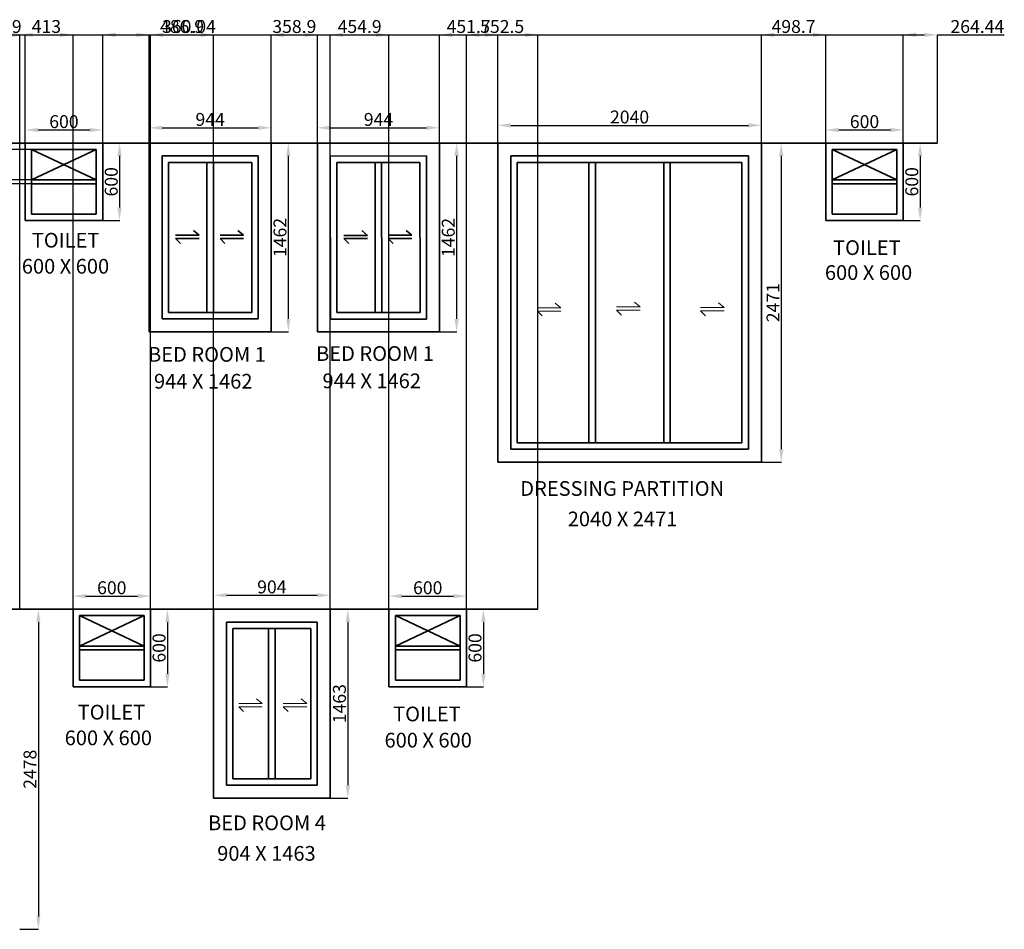
# Model space of a CAD drawing. Units: millimetres. Extents: x 5977 to 24120, y -1732 to 6209.
# Tile 3 of 3: x 16498 to 24120, y -1234 to 5807. Entities that reach past the tile are written whole.
import ezdxf

# ---------------------------------------------------------------- set-up
doc = ezdxf.new("R2010")
doc.units = ezdxf.units.MM
for name, color, linetype, lineweight in [('A-ANNO-DIMS', 2, 'Continuous', 18), ('A-ANNO-SYMB', 143, 'Continuous', 18), ('A-ANNO-TEXT', 7, 'Continuous', 25), ('A-GLAZ', 4, 'Continuous', 35)]:
    doc.layers.add(name, color=color, linetype=linetype, lineweight=lineweight)
doc.styles.get("Standard").update_dxf_attribs({"font": 'arial.ttf'})
doc.dimstyles.new('ISO-25', dxfattribs={"dimtxt": 100, "dimasz": 100, "dimexe": 1.25, "dimexo": 0.625, "dimtad": 1, "dimtxsty": 'Standard', "dimcen": 2.5, "dimadec": 0, "dimazin": 0, "dimtfac": 1, "dimtmove": 0, "dimatfit": 3, "dimfxl": 1, "dimarcsym": 0})

# ---------------------------------------------------------------- blocks, each defined once
blk = doc.blocks.new('*D11')
at = {"layer": 'A-ANNO-DIMS', "color": 0, "lineweight": -2, "transparency": 16777216}
for p, q in [((16540.9, 4852.8), (16540.9, 4954.6)), ((17140.9, 4852.8), (17140.9, 4954.6)), ((16640.9, 4953.4), (17040.9, 4953.4))]:
    blk.add_line(p, q, dxfattribs=at)
at = {"layer": 'A-ANNO-DIMS', "color": 0, "transparency": 16777216}
for points in [[(16640.9, 4970.1), (16640.9, 4936.7), (16540.9, 4953.4)], [(17040.9, 4970.1), (17040.9, 4936.7), (17140.9, 4953.4)]]:
    blk.add_solid(points, dxfattribs=at)
at = {"layer": 'Defpoints', "color": 0, "transparency": 16777216}
for p in [(17140.9, 4953.4), (16540.9, 4852.2), (17140.9, 4852.2)]:
    blk.add_point(p, dxfattribs=at)
at = {"layer": 'A-ANNO-DIMS', "color": 0, "transparency": 16777216, "insert": (16840.9, 5005.1), "char_height": 100, "attachment_point": 5}
blk.add_mtext('600', dxfattribs=at)
blk = doc.blocks.new('*D12')
at = {"layer": 'A-ANNO-DIMS', "color": 0, "lineweight": -2, "transparency": 16777216}
for p, q in [((17141.5, 4852.2), (17272.9, 4852.2)), ((17271.7, 4752.2), (17271.7, 4352.2)), ((17141.5, 4252.2), (17272.9, 4252.2))]:
    blk.add_line(p, q, dxfattribs=at)
at = {"layer": 'A-ANNO-DIMS', "color": 0, "transparency": 16777216}
for points in [[(17255, 4752.2), (17288.3, 4752.2), (17271.7, 4852.2)], [(17255, 4352.2), (17288.3, 4352.2), (17271.7, 4252.2)]]:
    blk.add_solid(points, dxfattribs=at)
at = {"layer": 'Defpoints', "color": 0, "transparency": 16777216}
for p in [(17140.9, 4852.2), (17140.9, 4252.2), (17271.7, 4252.2)]:
    blk.add_point(p, dxfattribs=at)
at = {"layer": 'A-ANNO-DIMS', "color": 0, "transparency": 16777216, "insert": (17220, 4552.2), "char_height": 100, "attachment_point": 5, "rotation": 90}
blk.add_mtext('600', dxfattribs=at)
blk = doc.blocks.new('*D13')
at = {"layer": 'A-ANNO-DIMS', "color": 0, "lineweight": -2, "transparency": 16777216}
for p, q in [((17500.9, 4852.8), (17500.9, 4971.3)), ((17600.9, 4970), (18344.9, 4970)), ((18444.9, 4852.8), (18444.9, 4971.3))]:
    blk.add_line(p, q, dxfattribs=at)
at = {"layer": 'A-ANNO-DIMS', "color": 0, "transparency": 16777216}
for points in [[(17600.9, 4986.7), (17600.9, 4953.4), (17500.9, 4970)], [(18344.9, 4986.7), (18344.9, 4953.4), (18444.9, 4970)]]:
    blk.add_solid(points, dxfattribs=at)
at = {"layer": 'Defpoints', "color": 0, "transparency": 16777216}
for p in [(18444.9, 4970), (17500.9, 4852.2), (18444.9, 4852.2)]:
    blk.add_point(p, dxfattribs=at)
at = {"layer": 'A-ANNO-DIMS', "color": 0, "transparency": 16777216, "insert": (17972.9, 5021.7), "char_height": 100, "attachment_point": 5}
blk.add_mtext('944', dxfattribs=at)
blk = doc.blocks.new('*D14')
at = {"layer": 'A-ANNO-DIMS', "color": 0, "lineweight": -2, "transparency": 16777216}
for p, q in [((18445.6, 4852.2), (18579.1, 4852.2)), ((18577.9, 4752.2), (18577.9, 3490.2)), ((18445.6, 3390.2), (18579.1, 3390.2))]:
    blk.add_line(p, q, dxfattribs=at)
at = {"layer": 'A-ANNO-DIMS', "color": 0, "transparency": 16777216}
for points in [[(18561.2, 4752.2), (18594.5, 4752.2), (18577.9, 4852.2)], [(18561.2, 3490.2), (18594.5, 3490.2), (18577.9, 3390.2)]]:
    blk.add_solid(points, dxfattribs=at)
at = {"layer": 'Defpoints', "color": 0, "transparency": 16777216}
for p in [(18444.9, 4852.2), (18444.9, 3390.2), (18577.9, 3390.2)]:
    blk.add_point(p, dxfattribs=at)
at = {"layer": 'A-ANNO-DIMS', "color": 0, "transparency": 16777216, "insert": (18526.2, 4121.2), "char_height": 100, "attachment_point": 5, "rotation": 90}
blk.add_mtext('1462', dxfattribs=at)
blk = doc.blocks.new('*D15')
at = {"layer": 'A-ANNO-DIMS', "color": 0, "lineweight": -2, "transparency": 16777216}
for p, q in [((18803.8, 4852.8), (18803.8, 4971.3)), ((18903.8, 4970), (19647.8, 4970)), ((19747.8, 4852.8), (19747.8, 4971.3))]:
    blk.add_line(p, q, dxfattribs=at)
at = {"layer": 'A-ANNO-DIMS', "color": 0, "transparency": 16777216}
for points in [[(18903.8, 4986.7), (18903.8, 4953.4), (18803.8, 4970)], [(19647.8, 4986.7), (19647.8, 4953.4), (19747.8, 4970)]]:
    blk.add_solid(points, dxfattribs=at)
at = {"layer": 'Defpoints', "color": 0, "transparency": 16777216}
for p in [(19747.8, 4970), (18803.8, 4852.2), (19747.8, 4852.2)]:
    blk.add_point(p, dxfattribs=at)
at = {"layer": 'A-ANNO-DIMS', "color": 0, "transparency": 16777216, "insert": (19275.8, 5021.7), "char_height": 100, "attachment_point": 5}
blk.add_mtext('944', dxfattribs=at)
blk = doc.blocks.new('*D16')
at = {"layer": 'A-ANNO-DIMS', "color": 0, "lineweight": -2, "transparency": 16777216}
for p, q in [((19748.5, 4852.2), (19882, 4852.2)), ((19880.8, 4752.2), (19880.8, 3490.2)), ((19748.5, 3390.2), (19882, 3390.2))]:
    blk.add_line(p, q, dxfattribs=at)
at = {"layer": 'A-ANNO-DIMS', "color": 0, "transparency": 16777216}
for points in [[(19864.1, 4752.2), (19897.4, 4752.2), (19880.8, 4852.2)], [(19864.1, 3490.2), (19897.4, 3490.2), (19880.8, 3390.2)]]:
    blk.add_solid(points, dxfattribs=at)
at = {"layer": 'Defpoints', "color": 0, "transparency": 16777216}
for p in [(19747.8, 4852.2), (19747.8, 3390.2), (19880.8, 3390.2)]:
    blk.add_point(p, dxfattribs=at)
at = {"layer": 'A-ANNO-DIMS', "color": 0, "transparency": 16777216, "insert": (19829.1, 4121.2), "char_height": 100, "attachment_point": 5, "rotation": 90}
blk.add_mtext('1462', dxfattribs=at)
blk = doc.blocks.new('*D17')
at = {"layer": 'A-ANNO-DIMS', "color": 0, "lineweight": -2, "transparency": 16777216}
for p, q in [((20199.5, 4852.8), (20199.5, 4990.3)), ((20299.5, 4989), (22139.5, 4989)), ((22239.5, 4852.8), (22239.5, 4990.3))]:
    blk.add_line(p, q, dxfattribs=at)
at = {"layer": 'A-ANNO-DIMS', "color": 0, "transparency": 16777216}
for points in [[(20299.5, 5005.7), (20299.5, 4972.4), (20199.5, 4989)], [(22139.5, 5005.7), (22139.5, 4972.4), (22239.5, 4989)]]:
    blk.add_solid(points, dxfattribs=at)
at = {"layer": 'Defpoints', "color": 0, "transparency": 16777216}
for p in [(22239.5, 4989), (20199.5, 4852.2), (22239.5, 4852.2)]:
    blk.add_point(p, dxfattribs=at)
at = {"layer": 'A-ANNO-DIMS', "color": 0, "transparency": 16777216, "insert": (21219.5, 5040.7), "char_height": 100, "attachment_point": 5}
blk.add_mtext('2040', dxfattribs=at)
blk = doc.blocks.new('*D18')
at = {"layer": 'A-ANNO-DIMS', "color": 0, "lineweight": -2, "transparency": 16777216}
for p, q in [((22240.1, 4852.2), (22394.9, 4852.2)), ((22393.6, 4752.2), (22393.6, 2481.2)), ((22240.1, 2381.2), (22394.9, 2381.2))]:
    blk.add_line(p, q, dxfattribs=at)
at = {"layer": 'A-ANNO-DIMS', "color": 0, "transparency": 16777216}
for points in [[(22377, 4752.2), (22410.3, 4752.2), (22393.6, 4852.2)], [(22377, 2481.2), (22410.3, 2481.2), (22393.6, 2381.2)]]:
    blk.add_solid(points, dxfattribs=at)
at = {"layer": 'Defpoints', "color": 0, "transparency": 16777216}
for p in [(22239.5, 4852.2), (22239.5, 2381.2), (22393.6, 2381.2)]:
    blk.add_point(p, dxfattribs=at)
at = {"layer": 'A-ANNO-DIMS', "color": 0, "transparency": 16777216, "insert": (22342.8, 3616.7), "char_height": 100, "attachment_point": 5, "rotation": 90}
blk.add_mtext('2471', dxfattribs=at)
blk = doc.blocks.new('*D19')
at = {"layer": 'A-ANNO-DIMS', "color": 0, "lineweight": -2, "transparency": 16777216}
for p, q in [((22738.2, 4852.8), (22738.2, 4954.6)), ((23338.2, 4852.8), (23338.2, 4954.6)), ((22838.2, 4953.4), (23238.2, 4953.4))]:
    blk.add_line(p, q, dxfattribs=at)
at = {"layer": 'A-ANNO-DIMS', "color": 0, "transparency": 16777216}
for points in [[(22838.2, 4970.1), (22838.2, 4936.7), (22738.2, 4953.4)], [(23238.2, 4970.1), (23238.2, 4936.7), (23338.2, 4953.4)]]:
    blk.add_solid(points, dxfattribs=at)
at = {"layer": 'Defpoints', "color": 0, "transparency": 16777216}
for p in [(23338.2, 4953.4), (22738.2, 4852.2), (23338.2, 4852.2)]:
    blk.add_point(p, dxfattribs=at)
at = {"layer": 'A-ANNO-DIMS', "color": 0, "transparency": 16777216, "insert": (23038.2, 5005.1), "char_height": 100, "attachment_point": 5}
blk.add_mtext('600', dxfattribs=at)
blk = doc.blocks.new('*D20')
at = {"layer": 'A-ANNO-DIMS', "color": 0, "lineweight": -2, "transparency": 16777216}
for p, q in [((23338.8, 4852.2), (23470.2, 4852.2)), ((23468.9, 4752.2), (23468.9, 4352.2)), ((23338.8, 4252.2), (23470.2, 4252.2))]:
    blk.add_line(p, q, dxfattribs=at)
at = {"layer": 'A-ANNO-DIMS', "color": 0, "transparency": 16777216}
for points in [[(23452.3, 4752.2), (23485.6, 4752.2), (23468.9, 4852.2)], [(23452.3, 4352.2), (23485.6, 4352.2), (23468.9, 4252.2)]]:
    blk.add_solid(points, dxfattribs=at)
at = {"layer": 'Defpoints', "color": 0, "transparency": 16777216}
for p in [(23338.2, 4852.2), (23338.2, 4252.2), (23468.9, 4252.2)]:
    blk.add_point(p, dxfattribs=at)
at = {"layer": 'A-ANNO-DIMS', "color": 0, "transparency": 16777216, "insert": (23417.2, 4552.2), "char_height": 100, "attachment_point": 5, "rotation": 90}
blk.add_mtext('600', dxfattribs=at)
blk = doc.blocks.new('*D25')
at = {"layer": 'A-ANNO-DIMS', "color": 0, "lineweight": -2, "transparency": 16777216}
for p, q in [((16911.4, 1244.3), (16911.4, 1346.1)), ((17011.4, 1344.9), (17411.4, 1344.9)), ((17511.4, 1244.3), (17511.4, 1346.1))]:
    blk.add_line(p, q, dxfattribs=at)
at = {"layer": 'A-ANNO-DIMS', "color": 0, "transparency": 16777216}
for points in [[(17011.4, 1361.5), (17011.4, 1328.2), (16911.4, 1344.9)], [(17411.4, 1361.5), (17411.4, 1328.2), (17511.4, 1344.9)]]:
    blk.add_solid(points, dxfattribs=at)
at = {"layer": 'Defpoints', "color": 0, "transparency": 16777216}
for p in [(17511.4, 1344.9), (16911.4, 1243.7), (17511.4, 1243.7)]:
    blk.add_point(p, dxfattribs=at)
at = {"layer": 'A-ANNO-DIMS', "color": 0, "transparency": 16777216, "insert": (17211.4, 1396.6), "char_height": 100, "attachment_point": 5}
blk.add_mtext('600', dxfattribs=at)
blk = doc.blocks.new('*D26')
at = {"layer": 'A-ANNO-DIMS', "color": 0, "lineweight": -2, "transparency": 16777216}
for p, q in [((17512.1, 1243.7), (17643.4, 1243.7)), ((17642.2, 1143.7), (17642.2, 743.7)), ((17512.1, 643.7), (17643.4, 643.7))]:
    blk.add_line(p, q, dxfattribs=at)
at = {"layer": 'A-ANNO-DIMS', "color": 0, "transparency": 16777216}
for points in [[(17625.5, 1143.7), (17658.9, 1143.7), (17642.2, 1243.7)], [(17625.5, 743.7), (17658.9, 743.7), (17642.2, 643.7)]]:
    blk.add_solid(points, dxfattribs=at)
at = {"layer": 'Defpoints', "color": 0, "transparency": 16777216}
for p in [(17511.4, 1243.7), (17511.4, 643.7), (17642.2, 643.7)]:
    blk.add_point(p, dxfattribs=at)
at = {"layer": 'A-ANNO-DIMS', "color": 0, "transparency": 16777216, "insert": (17590.5, 943.7), "char_height": 100, "attachment_point": 5, "rotation": 90}
blk.add_mtext('600', dxfattribs=at)
blk = doc.blocks.new('*D32')
at = {"layer": 'A-ANNO-DIMS', "color": 0, "lineweight": -2, "transparency": 16777216}
for p, q in [((16499.1, 1243.7), (16644.2, 1243.7)), ((16643, 1143.7), (16643, -1134.3)), ((16499.1, -1234.3), (16644.2, -1234.3))]:
    blk.add_line(p, q, dxfattribs=at)
at = {"layer": 'A-ANNO-DIMS', "color": 0, "transparency": 16777216}
for points in [[(16626.3, 1143.7), (16659.6, 1143.7), (16643, 1243.7)], [(16626.3, -1134.3), (16659.6, -1134.3), (16643, -1234.3)]]:
    blk.add_solid(points, dxfattribs=at)
at = {"layer": 'Defpoints', "color": 0, "transparency": 16777216}
for p in [(16498.5, 1243.7), (16498.5, -1234.3), (16643, -1234.3)]:
    blk.add_point(p, dxfattribs=at)
at = {"layer": 'A-ANNO-DIMS', "color": 0, "transparency": 16777216, "insert": (16591.3, 4.7), "char_height": 100, "attachment_point": 5, "rotation": 90}
blk.add_mtext('2478', dxfattribs=at)
blk = doc.blocks.new('*D33')
at = {"layer": 'A-ANNO-DIMS', "color": 0, "lineweight": -2, "transparency": 16777216}
for p, q in [((17998.3, 1244.3), (17998.3, 1352.8)), ((18098.3, 1351.6), (18802.3, 1351.6)), ((18902.3, 1244.3), (18902.3, 1352.8))]:
    blk.add_line(p, q, dxfattribs=at)
at = {"layer": 'A-ANNO-DIMS', "color": 0, "transparency": 16777216}
for points in [[(18098.3, 1368.3), (18098.3, 1334.9), (17998.3, 1351.6)], [(18802.3, 1368.3), (18802.3, 1334.9), (18902.3, 1351.6)]]:
    blk.add_solid(points, dxfattribs=at)
at = {"layer": 'Defpoints', "color": 0, "transparency": 16777216}
for p in [(18902.3, 1351.6), (17998.3, 1243.7), (18902.3, 1243.7)]:
    blk.add_point(p, dxfattribs=at)
at = {"layer": 'A-ANNO-DIMS', "color": 0, "transparency": 16777216, "insert": (18450.3, 1403.3), "char_height": 100, "attachment_point": 5}
blk.add_mtext('904', dxfattribs=at)
blk = doc.blocks.new('*D34')
at = {"layer": 'A-ANNO-DIMS', "color": 0, "lineweight": -2, "transparency": 16777216}
for p, q in [((18902.9, 1243.7), (19039.7, 1243.7)), ((19038.4, 1143.7), (19038.4, -119.3)), ((18902.9, -219.3), (19039.7, -219.3))]:
    blk.add_line(p, q, dxfattribs=at)
at = {"layer": 'A-ANNO-DIMS', "color": 0, "transparency": 16777216}
for points in [[(19021.7, 1143.7), (19055.1, 1143.7), (19038.4, 1243.7)], [(19021.7, -119.3), (19055.1, -119.3), (19038.4, -219.3)]]:
    blk.add_solid(points, dxfattribs=at)
at = {"layer": 'Defpoints', "color": 0, "transparency": 16777216}
for p in [(18902.3, 1243.7), (18902.3, -219.3), (19038.4, -219.3)]:
    blk.add_point(p, dxfattribs=at)
at = {"layer": 'A-ANNO-DIMS', "color": 0, "transparency": 16777216, "insert": (18986.7, 512.2), "char_height": 100, "attachment_point": 5, "rotation": 90}
blk.add_mtext('1463', dxfattribs=at)
blk = doc.blocks.new('*D35')
at = {"layer": 'A-ANNO-DIMS', "color": 0, "lineweight": -2, "transparency": 16777216}
for p, q in [((19357.2, 1244.3), (19357.2, 1346.1)), ((19457.2, 1344.9), (19857.2, 1344.9)), ((19957.2, 1244.3), (19957.2, 1346.1))]:
    blk.add_line(p, q, dxfattribs=at)
at = {"layer": 'A-ANNO-DIMS', "color": 0, "transparency": 16777216}
for points in [[(19457.2, 1361.5), (19457.2, 1328.2), (19357.2, 1344.9)], [(19857.2, 1361.5), (19857.2, 1328.2), (19957.2, 1344.9)]]:
    blk.add_solid(points, dxfattribs=at)
at = {"layer": 'Defpoints', "color": 0, "transparency": 16777216}
for p in [(19957.2, 1344.9), (19357.2, 1243.7), (19957.2, 1243.7)]:
    blk.add_point(p, dxfattribs=at)
at = {"layer": 'A-ANNO-DIMS', "color": 0, "transparency": 16777216, "insert": (19657.2, 1396.6), "char_height": 100, "attachment_point": 5}
blk.add_mtext('600', dxfattribs=at)
blk = doc.blocks.new('*D36')
at = {"layer": 'A-ANNO-DIMS', "color": 0, "lineweight": -2, "transparency": 16777216}
for p, q in [((19957.9, 1243.7), (20089.2, 1243.7)), ((20088, 1143.7), (20088, 743.7)), ((19957.9, 643.7), (20089.2, 643.7))]:
    blk.add_line(p, q, dxfattribs=at)
at = {"layer": 'A-ANNO-DIMS', "color": 0, "transparency": 16777216}
for points in [[(20071.3, 1143.7), (20104.7, 1143.7), (20088, 1243.7)], [(20071.3, 743.7), (20104.7, 743.7), (20088, 643.7)]]:
    blk.add_solid(points, dxfattribs=at)
at = {"layer": 'Defpoints', "color": 0, "transparency": 16777216}
for p in [(19957.2, 1243.7), (19957.2, 643.7), (20088, 643.7)]:
    blk.add_point(p, dxfattribs=at)
at = {"layer": 'A-ANNO-DIMS', "color": 0, "transparency": 16777216, "insert": (20036.3, 943.7), "char_height": 100, "attachment_point": 5, "rotation": 90}
blk.add_mtext('600', dxfattribs=at)
blk = doc.blocks.new('WIN-600x600-TOILET')
for p, q in [((16540.9, 4852.2), (16540.9, 4252.2)), ((16590.9, 4802.2), (16590.9, 4302.2)), ((16590.9, 4802.2), (17090.9, 4802.2)), ((16590.9, 4567.2), (17090.9, 4802.2)), ((17090.9, 4567.2), (16590.9, 4802.2)), ((17090.9, 4302.2), (17090.9, 4802.2)), ((17140.9, 4252.2), (17140.9, 4852.2)), ((16590.9, 4567.2), (17090.9, 4567.2)), ((16590.9, 4302.2), (17090.9, 4302.2)), ((16540.9, 4252.2), (17140.9, 4252.2))]:
    blk.add_line(p, q)
blk = doc.blocks.new('WIN-944x1462-BED')
for p, q in [((17600.9, 4752.2), (18344.9, 4752.2)), ((17600.9, 4752.2), (17600.9, 3490.2)), ((18344.9, 3490.2), (18344.9, 4752.2)), ((17650.9, 4702.2), (18294.9, 4702.2)), ((17650.9, 4702.2), (17650.9, 3540.2)), ((17947.9, 4702.2), (17947.9, 3540.2)), ((17997.9, 4702.2), (17997.9, 3540.2)), ((18294.9, 3540.2), (18294.9, 4702.2)), ((17705.1, 4138.2), (17887.8, 4138.2)), ((17887.8, 4138.2), (17843.7, 4175.4)), ((18049.1, 4138.2), (18231.8, 4138.2)), ((18231.8, 4138.2), (18187.7, 4175.4)), ((17705, 4113), (17887.4, 4113)), ((17705, 4113), (17742.7, 4075.4)), ((18049.1, 4113), (18231.4, 4113)), ((18049.1, 4113), (18086.7, 4075.4)), ((17650.9, 3540.2), (18294.9, 3540.2)), ((17600.9, 3490.2), (18344.9, 3490.2))]:
    blk.add_line(p, q)
blk = doc.blocks.new('ARROW-SLIDE')
for p, q in [((14721.8, 21.3), (14904.6, 21.3)), ((14904.6, 21.3), (14860.5, 58.6)), ((14721.8, -3.8), (14904.1, -3.8)), ((14721.8, -3.8), (14759.4, -41.4))]:
    blk.add_line(p, q)
blk = doc.blocks.new('*D41')
at = {"layer": 'A-ANNO-DIMS', "color": 0, "lineweight": -2, "transparency": 16777216}
for p, q in [((6975.8, 4852.8), (6975.8, 5690.9)), ((7075.8, 5689.7), (23502.6, 5689.7)), ((23602.6, 4852.8), (23602.6, 5690.9))]:
    blk.add_line(p, q, dxfattribs=at)
at = {"layer": 'A-ANNO-DIMS', "color": 0, "transparency": 16777216}
for points in [[(7075.8, 5706.3), (7075.8, 5673), (6975.8, 5689.7)], [(23502.6, 5706.3), (23502.6, 5673), (23602.6, 5689.7)]]:
    blk.add_solid(points, dxfattribs=at)
at = {"layer": 'Defpoints', "color": 0, "transparency": 16777216}
for p in [(23602.6, 5689.7), (6975.8, 4852.2), (23602.6, 4852.2)]:
    blk.add_point(p, dxfattribs=at)
at = {"layer": 'A-ANNO-DIMS', "color": 0, "transparency": 16777216, "insert": (15289.2, 5741.3), "char_height": 100, "attachment_point": 5}
blk.add_mtext('16627', dxfattribs=at)
blk = doc.blocks.new('*D42')
at = {"layer": 'A-ANNO-DIMS', "color": 0, "lineweight": -2, "transparency": 16777216}
for p, q in [((6931.9, 1244.3), (6931.9, 5690.9)), ((7031.9, 5689.7), (20409.7, 5689.7)), ((20509.7, 1244.3), (20509.7, 5690.9))]:
    blk.add_line(p, q, dxfattribs=at)
at = {"layer": 'A-ANNO-DIMS', "color": 0, "transparency": 16777216}
for points in [[(7031.9, 5706.3), (7031.9, 5673), (6931.9, 5689.7)], [(20409.7, 5706.3), (20409.7, 5673), (20509.7, 5689.7)]]:
    blk.add_solid(points, dxfattribs=at)
at = {"layer": 'Defpoints', "color": 0, "transparency": 16777216}
for p in [(20509.7, 5689.7), (6931.9, 1243.7), (20509.7, 1243.7)]:
    blk.add_point(p, dxfattribs=at)
at = {"layer": 'A-ANNO-DIMS', "color": 0, "transparency": 16777216, "insert": (13720.8, 5741.4), "char_height": 100, "attachment_point": 5}
blk.add_mtext('13578', dxfattribs=at)
blk = doc.blocks.new('*D48')
at = {"layer": 'A-ANNO-DIMS', "color": 0, "lineweight": -2, "transparency": 16777216}
for p, q in [((16145, 4852.8), (16145, 5690.9)), ((16245, 5689.7), (16440.9, 5689.7)), ((16540.9, 4852.8), (16540.9, 5690.9))]:
    blk.add_line(p, q, dxfattribs=at)
at = {"layer": 'A-ANNO-DIMS', "color": 0, "transparency": 16777216}
for points in [[(16245, 5706.3), (16245, 5673), (16145, 5689.7)], [(16440.9, 5706.3), (16440.9, 5673), (16540.9, 5689.7)]]:
    blk.add_solid(points, dxfattribs=at)
at = {"layer": 'Defpoints', "color": 0, "transparency": 16777216}
for p in [(16540.9, 5689.7), (16145, 4852.2), (16540.9, 4852.2)]:
    blk.add_point(p, dxfattribs=at)
at = {"layer": 'A-ANNO-DIMS', "color": 0, "transparency": 16777216, "insert": (16343, 5741.4), "char_height": 100, "attachment_point": 5}
blk.add_mtext('395.9', dxfattribs=at)
blk = doc.blocks.new('*D49')
at = {"layer": 'A-ANNO-DIMS', "color": 0, "lineweight": -2, "transparency": 16777216}
for p, q in [((17140.9, 4852.8), (17140.9, 5690.9)), ((17240.9, 5689.7), (17400.9, 5689.7)), ((17500.9, 4852.8), (17500.9, 5690.9)), ((17500.9, 5689.7), (18016.9, 5689.7))]:
    blk.add_line(p, q, dxfattribs=at)
at = {"layer": 'A-ANNO-DIMS', "color": 0, "transparency": 16777216}
for points in [[(17240.9, 5706.3), (17240.9, 5673), (17140.9, 5689.7)], [(17400.9, 5706.3), (17400.9, 5673), (17500.9, 5689.7)]]:
    blk.add_solid(points, dxfattribs=at)
at = {"layer": 'Defpoints', "color": 0, "transparency": 16777216}
for p in [(17500.9, 5689.7), (17140.9, 4852.2), (17500.9, 4852.2)]:
    blk.add_point(p, dxfattribs=at)
at = {"layer": 'A-ANNO-DIMS', "color": 0, "transparency": 16777216, "insert": (17808.9, 5741.4), "char_height": 100, "attachment_point": 5}
blk.add_mtext('360.04', dxfattribs=at)
blk = doc.blocks.new('*D50')
at = {"layer": 'A-ANNO-DIMS', "color": 0, "lineweight": -2, "transparency": 16777216}
for p, q in [((18444.9, 4852.8), (18444.9, 5690.9)), ((18544.9, 5689.7), (18703.8, 5689.7)), ((18803.8, 4852.8), (18803.8, 5690.9))]:
    blk.add_line(p, q, dxfattribs=at)
at = {"layer": 'A-ANNO-DIMS', "color": 0, "transparency": 16777216}
for points in [[(18544.9, 5706.3), (18544.9, 5673), (18444.9, 5689.7)], [(18703.8, 5706.3), (18703.8, 5673), (18803.8, 5689.7)]]:
    blk.add_solid(points, dxfattribs=at)
at = {"layer": 'Defpoints', "color": 0, "transparency": 16777216}
for p in [(18803.8, 5689.7), (18444.9, 4852.2), (18803.8, 4852.2)]:
    blk.add_point(p, dxfattribs=at)
at = {"layer": 'A-ANNO-DIMS', "color": 0, "transparency": 16777216, "insert": (18624.4, 5741.4), "char_height": 100, "attachment_point": 5}
blk.add_mtext('358.9', dxfattribs=at)
blk = doc.blocks.new('*D51')
at = {"layer": 'A-ANNO-DIMS', "color": 0, "lineweight": -2, "transparency": 16777216}
for p, q in [((19747.8, 4852.8), (19747.8, 5690.9)), ((19847.8, 5689.7), (20099.5, 5689.7)), ((20199.5, 4852.8), (20199.5, 5690.9))]:
    blk.add_line(p, q, dxfattribs=at)
at = {"layer": 'A-ANNO-DIMS', "color": 0, "transparency": 16777216}
for points in [[(19847.8, 5706.3), (19847.8, 5673), (19747.8, 5689.7)], [(20099.5, 5706.3), (20099.5, 5673), (20199.5, 5689.7)]]:
    blk.add_solid(points, dxfattribs=at)
at = {"layer": 'Defpoints', "color": 0, "transparency": 16777216}
for p in [(20199.5, 5689.7), (19747.8, 4852.2), (20199.5, 4852.2)]:
    blk.add_point(p, dxfattribs=at)
at = {"layer": 'A-ANNO-DIMS', "color": 0, "transparency": 16777216, "insert": (19973.7, 5741.3), "char_height": 100, "attachment_point": 5}
blk.add_mtext('451.7', dxfattribs=at)
blk = doc.blocks.new('*D52')
at = {"layer": 'A-ANNO-DIMS', "color": 0, "lineweight": -2, "transparency": 16777216}
for p, q in [((22239.5, 4852.8), (22239.5, 5690.9)), ((22339.5, 5689.7), (22638.2, 5689.7)), ((22738.2, 4852.8), (22738.2, 5690.9))]:
    blk.add_line(p, q, dxfattribs=at)
at = {"layer": 'A-ANNO-DIMS', "color": 0, "transparency": 16777216}
for points in [[(22339.5, 5706.3), (22339.5, 5673), (22239.5, 5689.7)], [(22638.2, 5706.3), (22638.2, 5673), (22738.2, 5689.7)]]:
    blk.add_solid(points, dxfattribs=at)
at = {"layer": 'Defpoints', "color": 0, "transparency": 16777216}
for p in [(22738.2, 5689.7), (22239.5, 4852.2), (22738.2, 4852.2)]:
    blk.add_point(p, dxfattribs=at)
at = {"layer": 'A-ANNO-DIMS', "color": 0, "transparency": 16777216, "insert": (22488.8, 5741.3), "char_height": 100, "attachment_point": 5}
blk.add_mtext('498.7', dxfattribs=at)
blk = doc.blocks.new('*D53')
at = {"layer": 'A-ANNO-DIMS', "color": 0, "lineweight": -2, "transparency": 16777216}
for p, q in [((23338.2, 4852.8), (23338.2, 5690.9)), ((23438.2, 5689.7), (23502.6, 5689.7)), ((23602.6, 4852.8), (23602.6, 5690.9)), ((23602.6, 5689.7), (24120.3, 5689.7))]:
    blk.add_line(p, q, dxfattribs=at)
at = {"layer": 'A-ANNO-DIMS', "color": 0, "transparency": 16777216}
for points in [[(23438.2, 5706.3), (23438.2, 5673), (23338.2, 5689.7)], [(23502.6, 5706.3), (23502.6, 5673), (23602.6, 5689.7)]]:
    blk.add_solid(points, dxfattribs=at)
at = {"layer": 'Defpoints', "color": 0, "transparency": 16777216}
for p in [(23602.6, 5689.7), (23338.2, 4852.2), (23602.6, 4852.2)]:
    blk.add_point(p, dxfattribs=at)
at = {"layer": 'A-ANNO-DIMS', "color": 0, "transparency": 16777216, "insert": (23911.5, 5741.3), "char_height": 100, "attachment_point": 5}
blk.add_mtext('264.44', dxfattribs=at)
blk = doc.blocks.new('*D57')
at = {"layer": 'A-ANNO-DIMS', "color": 0, "lineweight": -2, "transparency": 16777216}
for p, q in [((16498.5, 1244.3), (16498.5, 5690.9)), ((16598.5, 5689.7), (16811.4, 5689.7)), ((16911.4, 1244.3), (16911.4, 5690.9))]:
    blk.add_line(p, q, dxfattribs=at)
at = {"layer": 'A-ANNO-DIMS', "color": 0, "transparency": 16777216}
for points in [[(16598.5, 5706.3), (16598.5, 5673), (16498.5, 5689.7)], [(16811.4, 5706.3), (16811.4, 5673), (16911.4, 5689.7)]]:
    blk.add_solid(points, dxfattribs=at)
at = {"layer": 'Defpoints', "color": 0, "transparency": 16777216}
for p in [(16911.4, 5689.7), (16498.5, 1243.7), (16911.4, 1243.7)]:
    blk.add_point(p, dxfattribs=at)
at = {"layer": 'A-ANNO-DIMS', "color": 0, "transparency": 16777216, "insert": (16705, 5741.4), "char_height": 100, "attachment_point": 5}
blk.add_mtext('413', dxfattribs=at)
blk = doc.blocks.new('*D58')
at = {"layer": 'A-ANNO-DIMS', "color": 0, "lineweight": -2, "transparency": 16777216}
for p, q in [((17511.4, 1244.3), (17511.4, 5690.9)), ((17611.4, 5689.7), (17898.3, 5689.7)), ((17998.3, 1244.3), (17998.3, 5690.9))]:
    blk.add_line(p, q, dxfattribs=at)
at = {"layer": 'A-ANNO-DIMS', "color": 0, "transparency": 16777216}
for points in [[(17611.4, 5706.3), (17611.4, 5673), (17511.4, 5689.7)], [(17898.3, 5706.3), (17898.3, 5673), (17998.3, 5689.7)]]:
    blk.add_solid(points, dxfattribs=at)
at = {"layer": 'Defpoints', "color": 0, "transparency": 16777216}
for p in [(17998.3, 5689.7), (17511.4, 1243.7), (17998.3, 1243.7)]:
    blk.add_point(p, dxfattribs=at)
at = {"layer": 'A-ANNO-DIMS', "color": 0, "transparency": 16777216, "insert": (17754.9, 5741.3), "char_height": 100, "attachment_point": 5}
blk.add_mtext('486.9', dxfattribs=at)
blk = doc.blocks.new('*D59')
at = {"layer": 'A-ANNO-DIMS', "color": 0, "lineweight": -2, "transparency": 16777216}
for p, q in [((18902.3, 1244.3), (18902.3, 5690.9)), ((19002.3, 5689.7), (19257.2, 5689.7)), ((19357.2, 1244.3), (19357.2, 5690.9))]:
    blk.add_line(p, q, dxfattribs=at)
at = {"layer": 'A-ANNO-DIMS', "color": 0, "transparency": 16777216}
for points in [[(19002.3, 5706.3), (19002.3, 5673), (18902.3, 5689.7)], [(19257.2, 5706.3), (19257.2, 5673), (19357.2, 5689.7)]]:
    blk.add_solid(points, dxfattribs=at)
at = {"layer": 'Defpoints', "color": 0, "transparency": 16777216}
for p in [(19357.2, 5689.7), (18902.3, 1243.7), (19357.2, 1243.7)]:
    blk.add_point(p, dxfattribs=at)
at = {"layer": 'A-ANNO-DIMS', "color": 0, "transparency": 16777216, "insert": (19129.8, 5741.3), "char_height": 100, "attachment_point": 5}
blk.add_mtext('454.9', dxfattribs=at)
blk = doc.blocks.new('*D60')
at = {"layer": 'A-ANNO-DIMS', "color": 0, "lineweight": -2, "transparency": 16777216}
for p, q in [((19957.2, 1244.3), (19957.2, 5690.9)), ((20057.2, 5689.7), (20409.7, 5689.7)), ((20509.7, 1244.3), (20509.7, 5690.9))]:
    blk.add_line(p, q, dxfattribs=at)
at = {"layer": 'A-ANNO-DIMS', "color": 0, "transparency": 16777216}
for points in [[(20057.2, 5706.3), (20057.2, 5673), (19957.2, 5689.7)], [(20409.7, 5706.3), (20409.7, 5673), (20509.7, 5689.7)]]:
    blk.add_solid(points, dxfattribs=at)
at = {"layer": 'Defpoints', "color": 0, "transparency": 16777216}
for p in [(20509.7, 5689.7), (19957.2, 1243.7), (20509.7, 1243.7)]:
    blk.add_point(p, dxfattribs=at)
at = {"layer": 'A-ANNO-DIMS', "color": 0, "transparency": 16777216, "insert": (20233.5, 5741.3), "char_height": 100, "attachment_point": 5}
blk.add_mtext('552.5', dxfattribs=at)
blk = doc.blocks.new('*D67')
at = {"layer": 'A-ANNO-DIMS', "color": 0, "lineweight": -2, "transparency": 16777216}
for p, q in [((16590.3, 4802.2), (6093.2, 4802.2)), ((6094.4, 4702.2), (6094.4, 4667.2)), ((16590.3, 4567.2), (6093.2, 4567.2))]:
    blk.add_line(p, q, dxfattribs=at)
at = {"layer": 'A-ANNO-DIMS', "color": 0, "transparency": 16777216}
for points in [[(6077.8, 4702.2), (6111.1, 4702.2), (6094.4, 4802.2)], [(6077.8, 4667.2), (6111.1, 4667.2), (6094.4, 4567.2)]]:
    blk.add_solid(points, dxfattribs=at)
at = {"layer": 'Defpoints', "color": 0, "transparency": 16777216}
for p in [(16590.9, 4802.2), (6094.4, 4567.2), (16590.9, 4567.2)]:
    blk.add_point(p, dxfattribs=at)
at = {"layer": 'A-ANNO-DIMS', "color": 0, "transparency": 16777216, "insert": (6042.7, 4684.7), "char_height": 100, "attachment_point": 5, "rotation": 90}
blk.add_mtext('235', dxfattribs=at)
blk = doc.blocks.new('*D68')
at = {"layer": 'A-ANNO-DIMS', "color": 0, "lineweight": -2, "transparency": 16777216}
for p, q in [((6094.4, 4667.2), (6094.4, 4767.2)), ((16590.3, 4567.2), (6093.2, 4567.2)), ((16590.3, 4537.2), (6093.2, 4537.2)), ((6094.4, 4567.2), (6094.4, 4537.2)), ((6094.4, 4437.2), (6094.4, 4193.1))]:
    blk.add_line(p, q, dxfattribs=at)
at = {"layer": 'A-ANNO-DIMS', "color": 0, "transparency": 16777216}
for points in [[(6077.8, 4667.2), (6111.1, 4667.2), (6094.4, 4567.2)], [(6077.8, 4437.2), (6111.1, 4437.2), (6094.4, 4537.2)]]:
    blk.add_solid(points, dxfattribs=at)
at = {"layer": 'Defpoints', "color": 0, "transparency": 16777216}
for p in [(6094.4, 4537.2), (16590.9, 4567.2), (16590.9, 4537.2)]:
    blk.add_point(p, dxfattribs=at)
at = {"layer": 'A-ANNO-DIMS', "color": 0, "transparency": 16777216, "insert": (6042.7, 4265.1), "char_height": 100, "attachment_point": 5, "rotation": 90}
blk.add_mtext('30', dxfattribs=at)

msp = doc.modelspace()

# ---------------------------------------------------------------- linework, layer by layer
at = {"layer": 'A-GLAZ'}
for p, q in [((6975.757, 4852.16), (19747.827, 4852.16)), ((17500.947, 4852.16), (17500.947, 3390.16)), ((18444.947, 3390.16), (18444.947, 4852.16)), ((18803.827, 4852.16), (18803.827, 3390.16)), ((19747.827, 3390.16), (19747.827, 4852.16)), ((19747.827, 4852.16), (23602.612, 4852.16)), ((20199.487, 4852.16), (20199.487, 2381.16)), ((22239.487, 2381.16), (22239.487, 4852.16)), ((20299.487, 4752.16), (20299.487, 2481.16)), ((20299.487, 4752.16), (22139.487, 4752.16)), ((22139.487, 2481.16), (22139.487, 4752.16)), ((20349.487, 4702.16), (20349.487, 2531.16)), ((20349.487, 4702.16), (22089.487, 4702.16)), ((20904.487, 4702.16), (20904.487, 2531.16)), ((20954.487, 4702.16), (20954.487, 2531.16)), ((21484.487, 4702.16), (21484.487, 2531.16)), ((21534.487, 4702.16), (21534.487, 2531.16)), ((22089.487, 2531.16), (22089.487, 4702.16)), ((16590.904, 4537.16), (17090.904, 4537.16)), ((22788.171, 4537.16), (23288.171, 4537.16)), ((17500.947, 3390.16), (18444.947, 3390.16)), ((18803.827, 3390.16), (19747.827, 3390.16)), ((20349.487, 2531.16), (22089.487, 2531.16)), ((20299.487, 2481.16), (22139.487, 2481.16)), ((20199.487, 2381.16), (22239.487, 2381.16)), ((6931.935, 1243.651), (20509.687, 1243.651)), ((17998.29, 1243.651), (17998.29, -219.349)), ((18902.29, -219.349), (18902.29, 1243.651)), ((18098.29, 1143.651), (18802.29, 1143.651)), ((18098.29, 1143.651), (18098.29, -119.349)), ((18802.29, -119.349), (18802.29, 1143.651)), ((18148.29, 1093.651), (18752.29, 1093.651)), ((18148.29, 1093.651), (18148.29, -69.349)), ((18425.29, -69.349), (18425.29, 1093.651)), ((18475.29, -69.349), (18475.29, 1093.651)), ((18752.29, -69.349), (18752.29, 1093.651)), ((16961.436, 928.651), (17461.436, 928.651)), ((19407.232, 928.651), (19907.232, 928.651)), ((18148.29, -69.349), (18752.29, -69.349)), ((18098.29, -119.349), (18802.29, -119.349)), ((17998.29, -219.349), (18902.29, -219.349))]:
    msp.add_line(p, q, dxfattribs=at)

# ---------------------------------------------------------------- block references
at = {"layer": 'A-ANNO-SYMB'}
for p in [(5783.88, 3555.199), (6397.758, 3562.408), (7047.94, 3556.711), (3472.016, 492.379), (3816.033, 492.379)]:
    msp.add_blockref('ARROW-SLIDE', p, dxfattribs=at)
at = {"layer": 'A-GLAZ'}
for name, p in [('WIN-600x600-TOILET', (0, 0)), ('WIN-600x600-TOILET', (6197.267, 0)), ('WIN-944x1462-BED', (0, 0)), ('WIN-600x600-TOILET', (370.532, -3608.51)), ('WIN-600x600-TOILET', (2816.328, -3608.51))]:
    msp.add_blockref(name, p, dxfattribs=at)
at = {"layer": 'A-GLAZ', "rotation": 0.0459341649812088}
msp.add_blockref('WIN-944x1462-BED', (1305.814, -14.926), dxfattribs=at)

# ---------------------------------------------------------------- texts
at = {"layer": 'A-ANNO-TEXT'}
for s, height, p in [('TOILET', 113.8754, (16592.317, 4043.041)), ('TOILET', 113.8754, (22794.739, 3985.626)), ('600 X 600', 113.8754, (16514.983, 3841.299)), ('600 X 600', 113.8754, (22731.541, 3792.661)), ('BED ROOM 1', 113.8754, (18793.142, 3165.738)), ('BED ROOM 1', 113.8754, (17492.31, 3159.222)), ('944 X 1462', 113.8754, (17538.183, 2951.26)), ('944 X 1462', 113.8754, (18842.573, 2954.419)), ('DRESSING PARTITION', 113.87539, (20373.341, 2121.093)), ('2040 X 2471', 113.87539, (20740.99, 1885.315)), ('TOILET', 113.8754, (16947.217, 389.625)), ('TOILET', 113.8754, (19389.258, 375.751)), ('600 X 600', 113.8754, (16846.717, 190.714)), ('600 X 600', 113.8754, (19322.677, 173.015)), ('BED ROOM 4', 113.8754, (17956.978, -467.212)), ('904 X 1463', 113.8754, (18027.52, -703.48))]:
    msp.add_text(s, height=height, dxfattribs=at).set_placement(p)

# ---------------------------------------------------------------- dimensions: what is measured, and where the dimension line sits
at = {"layer": 'A-ANNO-DIMS'}
for base, p1, p2, override, picture, middle in [((20509.687, 5689.66), (6931.935, 1243.651), (20509.687, 1243.651), {"dimdec": 0, "dimlfac": 1, "dimrnd": 0, "dimzin": 0, "dimdsep": 46, "dimlunit": 2}, '*D42', (13720.811, 5741.377)), ((23602.612, 5689.66), (6975.757, 4852.16), (23602.612, 4852.16), {"dimdec": 0, "dimlfac": 1, "dimrnd": 0, "dimzin": 0, "dimdsep": 46, "dimlunit": 2}, '*D41', (15289.184, 5741.343)), ((16540.904, 5689.66), (16145.025, 4852.16), (16540.904, 4852.16), {"dimdec": 1, "dimlfac": 1, "dimrnd": 0, "dimzin": 0, "dimdsep": 46, "dimlunit": 2}, '*D48', (16342.964, 5741.377)), ((16911.436, 5689.66), (16498.47, 1243.651), (16911.436, 1243.651), {"dimdec": 0, "dimlfac": 1, "dimrnd": 0, "dimzin": 0, "dimdsep": 46, "dimlunit": 2}, '*D57', (16704.953, 5741.377)), ((17500.947, 5689.66), (17140.904, 4852.16), (17500.947, 4852.16), {"dimdec": 2, "dimlfac": 1, "dimrnd": 0, "dimzin": 0, "dimdsep": 46, "dimlunit": 2}, '*D49', (17808.904, 5741.377)), ((17998.29, 5689.66), (17511.436, 1243.651), (17998.29, 1243.651), {"dimdec": 1, "dimlfac": 1, "dimrnd": 0, "dimzin": 0, "dimdsep": 46, "dimlunit": 2}, '*D58', (17754.863, 5741.343)), ((18803.827, 5689.66), (18444.947, 4852.16), (18803.827, 4852.16), {"dimdec": 1, "dimlfac": 1, "dimrnd": 0, "dimzin": 0, "dimdsep": 46, "dimlunit": 2}, '*D50', (18624.387, 5741.377)), ((19357.232, 5689.66), (18902.29, 1243.651), (19357.232, 1243.651), {"dimdec": 1, "dimlfac": 1, "dimrnd": 0, "dimzin": 0, "dimdsep": 46, "dimlunit": 2}, '*D59', (19129.761, 5741.343)), ((20199.487, 5689.66), (19747.827, 4852.16), (20199.487, 4852.16), {"dimdec": 1, "dimlfac": 1, "dimrnd": 0, "dimzin": 0, "dimdsep": 46, "dimlunit": 2}, '*D51', (19973.657, 5741.343)), ((20509.687, 5689.66), (19957.232, 1243.651), (20509.687, 1243.651), {"dimdec": 1, "dimlfac": 1, "dimrnd": 0, "dimzin": 0, "dimdsep": 46, "dimlunit": 2}, '*D60', (20233.459, 5741.343)), ((22738.171, 5689.66), (22239.487, 4852.16), (22738.171, 4852.16), {"dimdec": 1, "dimlfac": 1, "dimrnd": 0, "dimzin": 0, "dimdsep": 46, "dimlunit": 2}, '*D52', (22488.829, 5741.343)), ((23602.612, 5689.66), (23338.171, 4852.16), (23602.612, 4852.16), {"dimdec": 2, "dimlfac": 1, "dimrnd": 0, "dimzin": 0, "dimdsep": 46, "dimlunit": 2}, '*D53', (23911.457, 5741.343)), ((17140.904, 4953.39), (16540.904, 4852.16), (17140.904, 4852.16), {"dimclrd": 0, "dimclre": 0, "dimclrt": 0}, '*D11', (16840.904, 5005.072)), ((18444.947, 4970.041), (17500.947, 4852.16), (18444.947, 4852.16), {"dimclrd": 0, "dimclre": 0, "dimclrt": 0}, '*D13', (17972.947, 5021.723)), ((19747.827, 4970.041), (18803.827, 4852.16), (19747.827, 4852.16), {"dimclrd": 0, "dimclre": 0, "dimclrt": 0}, '*D15', (19275.827, 5021.723)), ((22239.487, 4989.02), (20199.487, 4852.16), (22239.487, 4852.16), {"dimclrd": 0, "dimclre": 0, "dimclrt": 0}, '*D17', (21219.487, 5040.703)), ((23338.171, 4953.39), (22738.171, 4852.16), (23338.171, 4852.16), {"dimclrd": 0, "dimclre": 0, "dimclrt": 0}, '*D19', (23038.171, 5005.072)), ((17511.436, 1344.88), (16911.436, 1243.651), (17511.436, 1243.651), {"dimclrd": 0, "dimclre": 0, "dimclrt": 0}, '*D25', (17211.436, 1396.562)), ((18902.29, 1351.588), (17998.29, 1243.651), (18902.29, 1243.651), {"dimclrd": 0, "dimclre": 0, "dimclrt": 0}, '*D33', (18450.29, 1403.27)), ((19957.232, 1344.88), (19357.232, 1243.651), (19957.232, 1243.651), {"dimclrd": 0, "dimclre": 0, "dimclrt": 0}, '*D35', (19657.232, 1396.562))]:
    dim = msp.add_linear_dim(base=base, p1=p1, p2=p2, dimstyle='ISO-25', override=override, dxfattribs=at)
    dim.commit()
    dim.dimension.update_dxf_attribs({"geometry": picture, "text_midpoint": middle})
for base, p1, p2, override, picture, middle in [((6094.435, 4567.16), (16590.904, 4802.16), (16590.904, 4567.16), {"dimdec": 0, "dimlfac": 1, "dimrnd": 0, "dimzin": 0, "dimdsep": 46, "dimlunit": 2}, '*D67', (6042.718, 4684.66)), ((17271.665, 4252.16), (17140.904, 4852.16), (17140.904, 4252.16), {"dimclrd": 0, "dimclre": 0, "dimclrt": 0}, '*D12', (17219.982, 4552.16)), ((18577.878, 3390.16), (18444.947, 4852.16), (18444.947, 3390.16), {"dimclrd": 0, "dimclre": 0, "dimclrt": 0}, '*D14', (18526.196, 4121.16)), ((19880.759, 3390.16), (19747.827, 4852.16), (19747.827, 3390.16), {"dimclrd": 0, "dimclre": 0, "dimclrt": 0}, '*D16', (19829.077, 4121.16)), ((22393.618, 2381.16), (22239.487, 4852.16), (22239.487, 2381.16), {"dimclrd": 0, "dimclre": 0, "dimclrt": 0}, '*D18', (22342.788, 3616.66)), ((23468.931, 4252.16), (23338.171, 4852.16), (23338.171, 4252.16), {"dimclrd": 0, "dimclre": 0, "dimclrt": 0}, '*D20', (23417.249, 4552.16)), ((6094.435, 4537.16), (16590.904, 4567.16), (16590.904, 4537.16), {"dimdec": 0, "dimlfac": 1, "dimrnd": 0, "dimzin": 0, "dimdsep": 46, "dimlunit": 2}, '*D68', (6042.718, 4265.117)), ((16642.963, -1234.349), (16498.47, 1243.651), (16498.47, -1234.349), {"dimclrd": 0, "dimclre": 0, "dimclrt": 0}, '*D32', (16591.281, 4.651)), ((17642.197, 643.651), (17511.436, 1243.651), (17511.436, 643.651), {"dimclrd": 0, "dimclre": 0, "dimclrt": 0}, '*D26', (17590.514, 943.651)), ((19038.411, -219.349), (18902.29, 1243.651), (18902.29, -219.349), {"dimclrd": 0, "dimclre": 0, "dimclrt": 0}, '*D34', (18986.694, 512.151)), ((20087.992, 643.651), (19957.232, 1243.651), (19957.232, 643.651), {"dimclrd": 0, "dimclre": 0, "dimclrt": 0}, '*D36', (20036.31, 943.651))]:
    dim = msp.add_linear_dim(base=base, p1=p1, p2=p2, angle=90, dimstyle='ISO-25', override=override, dxfattribs=at)
    dim.commit()
    dim.dimension.update_dxf_attribs({"geometry": picture, "text_midpoint": middle})

doc.saveas('drawing.dxf')
